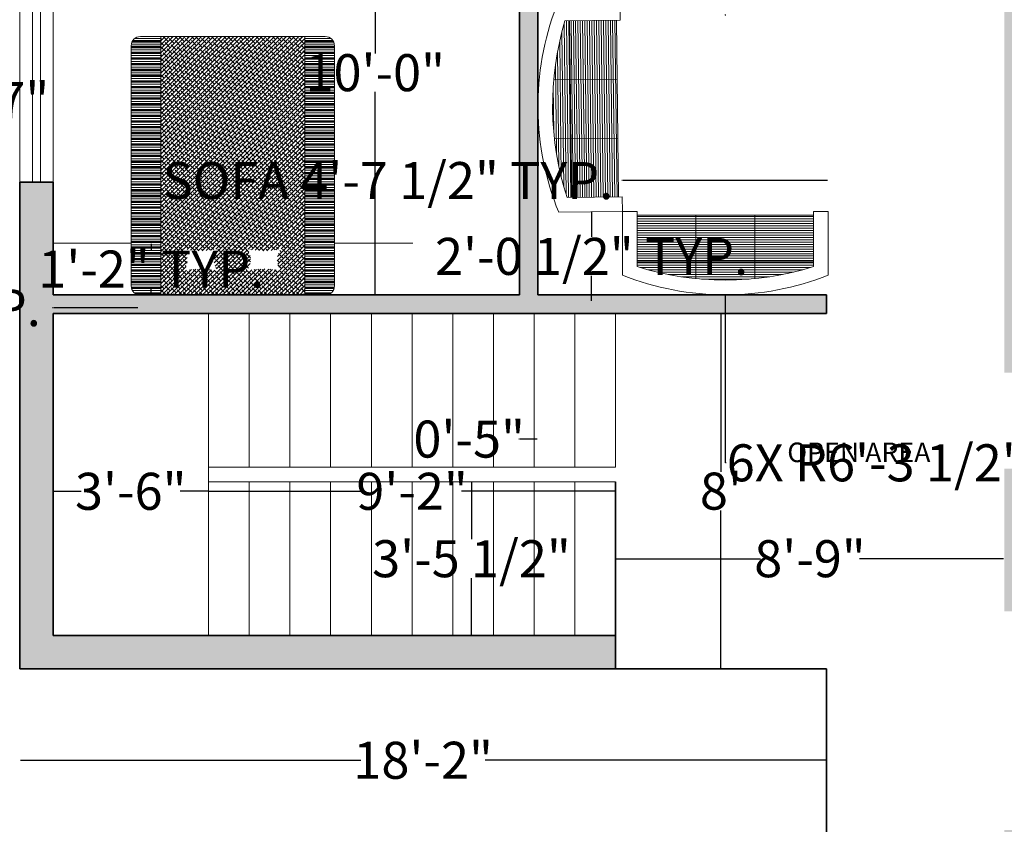
# Model space of a CAD drawing. Units: inches. Extents: x 1198 to 8596, y 144 to 930.
# Tile 3 of 5: x 1348 to 1614, y 536 to 753. Entities that reach past the tile are written whole.
import ezdxf

# ---------------------------------------------------------------- set-up
doc = ezdxf.new("R2010")
doc.units = ezdxf.units.IN
doc.header["$MEASUREMENT"] = 0
doc.layers.get('0').update_dxf_attribs({"color": 50})
for name, color, linetype, lineweight in [('A-ANNO-DIMS', 7, 'Continuous', 18), ('A-AREA-IDEN', 7, 'Continuous', 18), ('A-FLOR-STRS', 120, 'Continuous', 18), ('A-FURN', 11, 'Continuous', 18), ('A-FURN-PATT', 11, 'Continuous', 13), ('A-WALL-PATT', 150, 'Continuous', 13), ('WALL', 7, 'Continuous', 35), ('WINDOW', 2, 'Continuous', 18)]:
    doc.layers.add(name, color=color, linetype=linetype, lineweight=lineweight)
doc.styles.get("Standard").update_dxf_attribs({"font": 'arial.ttf'})
doc.dimstyles.get("Standard").update_dxf_attribs({"dimtxt": 10, "dimasz": 0.18, "dimexe": 0.18, "dimexo": 0.0625, "dimgap": 0.09, "dimtad": 0, "dimtih": 1, "dimtoh": 1, "dimdec": 0, "dimzin": 0, "dimdsep": 46, "dimlunit": 3, "dimtxsty": 'Standard', "dimcen": 0.09, "dimse1": 1, "dimse2": 1, "dimadec": 0, "dimazin": 0, "dimtfac": 1, "dimtdec": 0, "dimtofl": 0, "dimtmove": 0, "dimatfit": 3, "dimfxl": 1, "dimtolj": 1, "dimtzin": 0, "dimarcsym": 0})

# ---------------------------------------------------------------- blocks, each defined once
blk = doc.blocks.new('*D2')
at = {"layer": 'A-ANNO-DIMS', "color": 0, "lineweight": -2, "transparency": 16777216}
for p, q in [((1509.07, 607.65), (1548, 607.65)), ((1613.71, 607.65), (1574.77, 607.65))]:
    blk.add_line(p, q, dxfattribs=at)
at = {"layer": 'A-ANNO-DIMS', "color": 0, "transparency": 16777216}
for points in [[(1509.07, 607.68), (1509.07, 607.62), (1508.89, 607.65)], [(1613.71, 607.68), (1613.71, 607.62), (1613.89, 607.65)]]:
    blk.add_solid(points, dxfattribs=at)
at = {"layer": 'Defpoints', "color": 0, "transparency": 16777216}
for p in [(1508.89, 607.65), (1613.89, 607.65), (1613.89, 607.65)]:
    blk.add_point(p, dxfattribs=at)
at = {"layer": 'A-ANNO-DIMS', "color": 0, "transparency": 16777216, "insert": (1561.39, 607.65), "char_height": 10, "attachment_point": 5}
blk.add_mtext('\\A1;8\'-9"', dxfattribs=at)
blk = doc.blocks.new('*D3')
at = {"layer": 'A-ANNO-DIMS', "color": 0, "lineweight": -2, "transparency": 16777216}
for p, q in [((1537.33, 673.72), (1537.33, 631.09)), ((1537.33, 578.08), (1537.33, 620.7))]:
    blk.add_line(p, q, dxfattribs=at)
at = {"layer": 'A-ANNO-DIMS', "color": 0, "transparency": 16777216}
for points in [[(1537.3, 673.72), (1537.36, 673.72), (1537.33, 673.9)], [(1537.3, 578.08), (1537.36, 578.08), (1537.33, 577.9)]]:
    blk.add_solid(points, dxfattribs=at)
at = {"layer": 'Defpoints', "color": 0, "transparency": 16777216}
for p in [(1537.33, 673.9), (1537.33, 577.9), (1537.33, 577.9)]:
    blk.add_point(p, dxfattribs=at)
at = {"layer": 'A-ANNO-DIMS', "color": 0, "transparency": 16777216, "insert": (1537.33, 625.9), "char_height": 10, "attachment_point": 5}
blk.add_mtext("\\A1;8'", dxfattribs=at)
blk = doc.blocks.new('WD_WIN4')
for p, q in [((-0.5, 0.5), (0.5, 0.5)), ((-0.5, 0.12), (0.5, 0.12)), ((-0.5, -0.12), (0.5, -0.12)), ((-0.5, -0.5), (0.5, -0.5))]:
    blk.add_line(p, q)
blk = doc.blocks.new('Sofa - Roundback 7 ft.')
for p, q in [((-12.00002, -32.4421), (-12.00003, -6.5971)), ((11.99997, -32.4421), (11.99998, -6.5971)), ((-36.000027, -34), (-36.000027, -11.4696)), ((35.99998, -34), (35.99998, -11.4696)), ((-35.999844, -13.3819), (35.9998, -13.3819)), ((-36.000027, -32.4421), (35.99998, -32.4421))]:
    blk.add_line(p, q)
for points in [[(-36.000027, -34), (-42.000027, -34), (-42.000027, -8)], [(41.99998, -8), (41.99998, -34), (35.99998, -34)]]:
    blk.add_lwpolyline(points)
for centre, radius, start, end in [((0, -114.25), 114.25, 68.43141, 111.5686), ((-0.00001, -127.1968), 121.1968, 72.72033, 107.2797)]:
    blk.add_arc(centre, radius, start, end)
blk = doc.blocks.new('*D16')
at = {"layer": 'A-ANNO-DIMS', "color": 0, "lineweight": -2, "transparency": 16777216}
for p, q in [((1337.03, 884.72), (1337.03, 736.59)), ((1337.03, 578.08), (1337.03, 726.2))]:
    blk.add_line(p, q, dxfattribs=at)
at = {"layer": 'A-ANNO-DIMS', "color": 0, "transparency": 16777216}
for points in [[(1337, 884.72), (1337.06, 884.72), (1337.03, 884.9)], [(1337, 578.08), (1337.06, 578.08), (1337.03, 577.9)]]:
    blk.add_solid(points, dxfattribs=at)
at = {"layer": 'Defpoints', "color": 0, "transparency": 16777216}
for p in [(1347.89, 884.9), (1337.03, 577.9), (1347.89, 577.9)]:
    blk.add_point(p, dxfattribs=at)
at = {"layer": 'A-ANNO-DIMS', "color": 0, "transparency": 16777216, "insert": (1337.03, 731.4), "char_height": 10, "attachment_point": 5}
blk.add_mtext('\\A1;25\'-7"', dxfattribs=at)
blk = doc.blocks.new('*D17')
at = {"layer": 'A-ANNO-DIMS', "color": 0, "lineweight": -2, "transparency": 16777216}
for p, q in [((1288.75, 884.72), (1288.75, 551.09)), ((1288.75, 207.08), (1288.75, 540.7))]:
    blk.add_line(p, q, dxfattribs=at)
at = {"layer": 'A-ANNO-DIMS', "color": 0, "transparency": 16777216}
for points in [[(1288.72, 884.72), (1288.78, 884.72), (1288.75, 884.9)], [(1288.72, 207.08), (1288.78, 207.08), (1288.75, 206.9)]]:
    blk.add_solid(points, dxfattribs=at)
at = {"layer": 'Defpoints', "color": 0, "transparency": 16777216}
for p in [(1347.89, 884.9), (1288.75, 206.9), (1347.89, 206.9)]:
    blk.add_point(p, dxfattribs=at)
at = {"layer": 'A-ANNO-DIMS', "color": 0, "transparency": 16777216, "insert": (1288.75, 545.9), "char_height": 10, "attachment_point": 5}
blk.add_mtext('\\A1;56\'-6"', dxfattribs=at)
blk = doc.blocks.new('*D18')
at = {"layer": 'A-ANNO-DIMS', "color": 0, "lineweight": -2, "transparency": 16777216}
for p, q in [((1348.07, 553.22), (1440.09, 553.22)), ((1565.71, 553.22), (1473.68, 553.22))]:
    blk.add_line(p, q, dxfattribs=at)
at = {"layer": 'A-ANNO-DIMS', "color": 0, "transparency": 16777216}
for points in [[(1348.07, 553.25), (1348.07, 553.19), (1347.89, 553.22)], [(1565.71, 553.25), (1565.71, 553.19), (1565.89, 553.22)]]:
    blk.add_solid(points, dxfattribs=at)
at = {"layer": 'Defpoints', "color": 0, "transparency": 16777216}
for p in [(1347.89, 577.9), (1565.89, 577.9), (1565.89, 553.22)]:
    blk.add_point(p, dxfattribs=at)
at = {"layer": 'A-ANNO-DIMS', "color": 0, "transparency": 16777216, "insert": (1456.89, 553.22), "char_height": 10, "attachment_point": 5}
blk.add_mtext('\\A1;18\'-2"', dxfattribs=at)
blk = doc.blocks.new('NIGHTSTAND')
for p, q in [((23.07, 13.96), (0, 13.96)), ((23.07, 0), (23.07, 13.96)), ((1.94, 0), (23.07, 0))]:
    blk.add_line(p, q)
blk = doc.blocks.new('*D26')
at = {"layer": 'A-ANNO-DIMS', "color": 0, "lineweight": -2, "transparency": 16777216}
for p, q in [((1510.72, 709.76), (1510.54, 709.76)), ((1566.15, 709.76), (1510.9, 709.76))]:
    blk.add_line(p, q, dxfattribs=at)
at = {"layer": 'A-ANNO-DIMS', "color": 0, "transparency": 16777216}
for points in [[(1510.9, 709.79), (1510.9, 709.73), (1510.72, 709.76)], [(1566.15, 709.79), (1566.15, 709.73), (1566.33, 709.76)]]:
    blk.add_solid(points, dxfattribs=at)
at = {"layer": 'Defpoints', "color": 0, "transparency": 16777216}
for p in [(1510.72, 709.76), (1510.72, 701.42), (1566.33, 701.42)]:
    blk.add_point(p, dxfattribs=at)
at = {"layer": 'A-ANNO-DIMS', "color": 0, "transparency": 16777216, "insert": (1447.39, 709.76), "char_height": 10, "attachment_point": 5}
blk.add_mtext('\\A1;SOFA 4\'-7 1/2" TYP.', dxfattribs=at)
blk = doc.blocks.new('*D27')
at = {"layer": 'A-ANNO-DIMS', "color": 0, "lineweight": -2, "transparency": 16777216}
for p, q in [((1502.38, 701.24), (1502.38, 694.55)), ((1502.38, 677.33), (1502.38, 684.03))]:
    blk.add_line(p, q, dxfattribs=at)
at = {"layer": 'A-ANNO-DIMS', "color": 0, "transparency": 16777216}
for points in [[(1502.35, 701.24), (1502.41, 701.24), (1502.38, 701.42)], [(1502.35, 677.33), (1502.41, 677.33), (1502.38, 677.15)]]:
    blk.add_solid(points, dxfattribs=at)
at = {"layer": 'Defpoints', "color": 0, "transparency": 16777216}
for p in [(1510.72, 701.42), (1502.38, 677.15), (1510.72, 677.15)]:
    blk.add_point(p, dxfattribs=at)
at = {"layer": 'A-ANNO-DIMS', "color": 0, "transparency": 16777216, "insert": (1502.38, 689.29), "char_height": 10, "attachment_point": 5}
blk.add_mtext('\\A1;2\'-0 1/2" TYP.', dxfattribs=at)
blk = doc.blocks.new('*D28')
at = {"layer": 'A-ANNO-DIMS', "color": 0, "lineweight": -2, "transparency": 16777216}
for p, q in [((1356.89, 675.44), (1356.71, 675.44)), ((1379.78, 675.44), (1357.07, 675.44))]:
    blk.add_line(p, q, dxfattribs=at)
at = {"layer": 'A-ANNO-DIMS', "color": 0, "transparency": 16777216}
for points in [[(1357.07, 675.47), (1357.07, 675.41), (1356.89, 675.44)], [(1379.78, 675.47), (1379.78, 675.41), (1379.96, 675.44)]]:
    blk.add_solid(points, dxfattribs=at)
at = {"layer": 'Defpoints', "color": 0, "transparency": 16777216}
for p in [(1356.89, 678.9), (1379.96, 678.9), (1356.89, 675.44)]:
    blk.add_point(p, dxfattribs=at)
at = {"layer": 'A-ANNO-DIMS', "color": 0, "transparency": 16777216, "insert": (1275.15, 675.44), "char_height": 10, "attachment_point": 5}
blk.add_mtext('\\A1;NIGHTSTAND 1\'-11" TYP.', dxfattribs=at)
blk = doc.blocks.new('*D29')
at = {"layer": 'A-ANNO-DIMS', "color": 0, "lineweight": -2, "transparency": 16777216}
for p, q in [((1383.42, 692.67), (1383.42, 690.99)), ((1383.42, 679.08), (1383.42, 680.76))]:
    blk.add_line(p, q, dxfattribs=at)
at = {"layer": 'A-ANNO-DIMS', "color": 0, "transparency": 16777216}
for points in [[(1383.39, 692.67), (1383.45, 692.67), (1383.42, 692.85)], [(1383.39, 679.08), (1383.45, 679.08), (1383.42, 678.9)]]:
    blk.add_solid(points, dxfattribs=at)
at = {"layer": 'Defpoints', "color": 0, "transparency": 16777216}
for p in [(1379.96, 692.85), (1379.96, 678.9), (1383.42, 678.9)]:
    blk.add_point(p, dxfattribs=at)
at = {"layer": 'A-ANNO-DIMS', "color": 0, "transparency": 16777216, "insert": (1383.42, 685.87), "char_height": 10, "attachment_point": 5}
blk.add_mtext('\\A1;1\'-2" TYP.', dxfattribs=at)
blk = doc.blocks.new('*D38')
at = {"layer": 'A-ANNO-DIMS', "color": 0, "lineweight": -2, "transparency": 16777216}
for p, q in [((1443.94, 798.72), (1443.94, 744.09)), ((1443.94, 679.08), (1443.94, 733.7))]:
    blk.add_line(p, q, dxfattribs=at)
at = {"layer": 'A-ANNO-DIMS', "color": 0, "transparency": 16777216}
for points in [[(1443.91, 798.72), (1443.97, 798.72), (1443.94, 798.9)], [(1443.91, 679.08), (1443.97, 679.08), (1443.94, 678.9)]]:
    blk.add_solid(points, dxfattribs=at)
at = {"layer": 'Defpoints', "color": 0, "transparency": 16777216}
for p in [(1443.94, 798.9), (1482.89, 798.9), (1482.89, 678.9)]:
    blk.add_point(p, dxfattribs=at)
at = {"layer": 'A-ANNO-DIMS', "color": 0, "transparency": 16777216, "insert": (1443.94, 738.9), "char_height": 10, "attachment_point": 5}
blk.add_mtext('\\A1;10\'-0"', dxfattribs=at)
blk = doc.blocks.new('*D39')
at = {"layer": 'A-ANNO-DIMS', "color": 0, "lineweight": -2, "transparency": 16777216}
for p, q in [((1399.07, 625.85), (1440.5, 625.85)), ((1508.71, 625.85), (1467.27, 625.85))]:
    blk.add_line(p, q, dxfattribs=at)
at = {"layer": 'A-ANNO-DIMS', "color": 0, "transparency": 16777216}
for points in [[(1399.07, 625.88), (1399.07, 625.82), (1398.89, 625.85)], [(1508.71, 625.88), (1508.71, 625.82), (1508.89, 625.85)]]:
    blk.add_solid(points, dxfattribs=at)
at = {"layer": 'Defpoints', "color": 0, "transparency": 16777216}
for p in [(1508.89, 625.85), (1398.89, 586.9), (1508.89, 586.9)]:
    blk.add_point(p, dxfattribs=at)
at = {"layer": 'A-ANNO-DIMS', "color": 0, "transparency": 16777216, "insert": (1453.89, 625.85), "char_height": 10, "attachment_point": 5}
blk.add_mtext('\\A1;9\'-2"', dxfattribs=at)
blk = doc.blocks.new('*D40')
at = {"layer": 'A-ANNO-DIMS', "color": 0, "lineweight": -2, "transparency": 16777216}
for p, q in [((1357.07, 625.85), (1364.51, 625.85)), ((1398.71, 625.85), (1391.26, 625.85))]:
    blk.add_line(p, q, dxfattribs=at)
at = {"layer": 'A-ANNO-DIMS', "color": 0, "transparency": 16777216}
for points in [[(1357.07, 625.88), (1357.07, 625.82), (1356.89, 625.85)], [(1398.71, 625.88), (1398.71, 625.82), (1398.89, 625.85)]]:
    blk.add_solid(points, dxfattribs=at)
at = {"layer": 'Defpoints', "color": 0, "transparency": 16777216}
for p in [(1398.89, 625.85), (1356.89, 586.9), (1398.89, 586.9)]:
    blk.add_point(p, dxfattribs=at)
at = {"layer": 'A-ANNO-DIMS', "color": 0, "transparency": 16777216, "insert": (1377.89, 625.85), "char_height": 10, "attachment_point": 5}
blk.add_mtext('\\A1;3\'-6"', dxfattribs=at)
blk = doc.blocks.new('*D41')
at = {"layer": 'A-ANNO-DIMS', "color": 0, "lineweight": -2, "transparency": 16777216}
for p, q in [((1469.94, 628.22), (1469.94, 612.91)), ((1469.94, 587.08), (1469.94, 602.38))]:
    blk.add_line(p, q, dxfattribs=at)
at = {"layer": 'A-ANNO-DIMS', "color": 0, "transparency": 16777216}
for points in [[(1469.91, 628.22), (1469.97, 628.22), (1469.94, 628.4)], [(1469.91, 587.08), (1469.97, 587.08), (1469.94, 586.9)]]:
    blk.add_solid(points, dxfattribs=at)
at = {"layer": 'Defpoints', "color": 0, "transparency": 16777216}
for p in [(1469.94, 628.4), (1508.89, 628.4), (1508.89, 586.9)]:
    blk.add_point(p, dxfattribs=at)
at = {"layer": 'A-ANNO-DIMS', "color": 0, "transparency": 16777216, "insert": (1469.94, 607.65), "char_height": 10, "attachment_point": 5}
blk.add_mtext('\\A1;3\'-5 1/2"', dxfattribs=at)
blk = doc.blocks.new('*D54')
at = {"layer": 'A-ANNO-DIMS', "color": 0, "lineweight": -2, "transparency": 16777216}
for p, q in [((1308.94, 626.78), (1308.94, 597.25)), ((1308.94, 557.33), (1308.94, 586.85))]:
    blk.add_line(p, q, dxfattribs=at)
at = {"layer": 'A-ANNO-DIMS', "color": 0, "transparency": 16777216}
for points in [[(1308.91, 626.78), (1308.97, 626.78), (1308.94, 626.96)], [(1308.91, 557.33), (1308.97, 557.33), (1308.94, 557.15)]]:
    blk.add_solid(points, dxfattribs=at)
at = {"layer": 'Defpoints', "color": 0, "transparency": 16777216}
for p in [(1308.94, 626.96), (1802.33, 626.96), (1802.33, 557.15)]:
    blk.add_point(p, dxfattribs=at)
at = {"layer": 'A-ANNO-DIMS', "color": 0, "transparency": 16777216, "insert": (1308.94, 592.05), "char_height": 10, "attachment_point": 5}
blk.add_mtext('\\A1;5\'-10"', dxfattribs=at)
blk = doc.blocks.new('*D68')
at = {"layer": 'A-ANNO-DIMS', "color": 0, "lineweight": -2, "transparency": 16777216}
for p, q in [((1482.89, 639.95), (1482.71, 639.95)), ((1487.71, 639.95), (1483.07, 639.95))]:
    blk.add_line(p, q, dxfattribs=at)
at = {"layer": 'A-ANNO-DIMS', "color": 0, "transparency": 16777216}
for points in [[(1483.07, 639.98), (1483.07, 639.92), (1482.89, 639.95)], [(1487.71, 639.98), (1487.71, 639.92), (1487.89, 639.95)]]:
    blk.add_solid(points, dxfattribs=at)
at = {"layer": 'Defpoints', "color": 0, "transparency": 16777216}
for p in [(1482.89, 678.9), (1487.89, 678.9), (1482.89, 639.95)]:
    blk.add_point(p, dxfattribs=at)
at = {"layer": 'A-ANNO-DIMS', "color": 0, "transparency": 16777216, "insert": (1469.32, 639.95), "char_height": 10, "attachment_point": 5}
blk.add_mtext('\\A1;0\'-5"', dxfattribs=at)
blk = doc.blocks.new('*D69')
at = {"layer": 'A-ANNO-DIMS', "color": 0, "lineweight": -2, "transparency": 16777216}
for p, q in [((1538.43, 754.55), (1538.61, 754.55)), ((1538.52, 754.46), (1538.52, 754.64)), ((1538.53, 633.54), (1538.53, 678.74)), ((1538.71, 633.54), (1538.53, 633.54))]:
    blk.add_line(p, q, dxfattribs=at)
at = {"layer": 'A-ANNO-DIMS', "color": 0, "transparency": 16777216}
blk.add_solid([(1538.56, 678.74), (1538.5, 678.74), (1538.53, 678.92)], dxfattribs=at)
at = {"layer": 'Defpoints', "color": 0, "transparency": 16777216}
for p in [(1538.52, 754.55), (1538.53, 678.92)]:
    blk.add_point(p, dxfattribs=at)
at = {"layer": 'A-ANNO-DIMS', "color": 0, "transparency": 16777216, "insert": (1579.29, 633.54), "char_height": 10, "attachment_point": 5}
blk.add_mtext('\\A1;6X R6\'-3 1/2"', dxfattribs=at)

msp = doc.modelspace()

# ---------------------------------------------------------------- hatches: boundary and pattern name
at = {"layer": 'A-FURN-PATT'}
h = msp.add_hatch(dxfattribs=at)
h.set_pattern_fill('LINE', color=256, scale=5, angle=-89.3197)
h.set_pattern_definition([(270.6803, (790.78874, 2257.74066), (0.62495594, 0.00742075), [])])
h.paths.add_polyline_path([(1509.27, 737.14), (1509.08, 753.02), (1496.46, 752.87), (1496.65, 736.99)])
h.paths.add_polyline_path([(1509.46, 721.25), (1509.27, 737.14), (1496.65, 736.99), (1496.84, 721.1)])
h.paths.add_polyline_path([(1509.64, 705.36), (1509.46, 721.25), (1496.84, 721.1), (1497.03, 705.21)])
h.paths.add_polyline_path([(1495.76, 705.2), (1497.03, 705.21), (1496.84, 721.1), (1492.35, 721.05, 0.050647)])
h.paths.add_polyline_path([(1496.84, 721.1), (1496.65, 736.99), (1492.16, 736.93, 0.049628), (1492.35, 721.05)])
h.paths.add_polyline_path([(1496.65, 736.99), (1496.46, 752.87), (1495.2, 752.86, 0.050647), (1492.16, 736.93)])
h = msp.add_hatch(dxfattribs=at)
h.set_pattern_fill('PLASTI', color=256, scale=6.190048)
h.set_pattern_definition([(0, (104.9537, 267.4466), (0, 1.547512), []), (0, (104.9537, 267.64), (0, 1.547512), []), (0, (104.9537, 267.8335), (0, 1.547512), []), (0, (104.9537, 268.4138), (0, 1.547512), [])])
h.paths.add_polyline_path([(1424.95, 678.84), (1430.45, 678.84, 0.414214), (1432.92, 681.31), (1432.92, 746.17, 0.414214), (1430.45, 748.65), (1424.95, 748.65)])
h.paths.add_polyline_path([(1378.02, 681.31, 0.414214), (1380.5, 678.84), (1386, 678.84), (1386, 748.65), (1380.5, 748.65, 0.414214), (1378.02, 746.17)])
h = msp.add_hatch(dxfattribs=at)
h.set_pattern_fill('ANSI38', color=256, scale=6.190048)
h.set_pattern_definition([(45, (104.9537, 267.4466), (-0.5471281, 0.5471281), []), (135, (104.9537, 267.4466), (-1.6413843, 0.5471281), [1.93439, -1.160634])])
h.paths.add_polyline_path([(1386, 678.84), (1424.95, 678.84), (1424.95, 748.65), (1386, 748.65)])
h.paths.add_polyline_path([(1401.43, 691.35, 0.358285), (1401.43, 685.35, 0.116256), (1392.11, 685.35, 0.358285), (1392.11, 691.35, 0.116256)], flags=16)
h.paths.add_polyline_path([(1409.19, 691.35, 0.116256), (1418.51, 691.35, 0.358285), (1418.51, 685.35, 0.116256), (1409.19, 685.35, 0.358285)], flags=16)
h = msp.add_hatch(dxfattribs=at)
h.set_pattern_fill('LINE', color=256, scale=5)
h.set_pattern_definition([(0, (1.553, 0.01844), (0, 0.625), [])])
h.paths.add_polyline_path([(1530.58, 700.39), (1514.69, 700.39), (1514.69, 687.77), (1530.58, 687.77)])
h.paths.add_polyline_path([(1546.47, 700.39), (1530.58, 700.39), (1530.58, 687.77), (1546.47, 687.77)])
h.paths.add_polyline_path([(1562.36, 700.39), (1546.47, 700.39), (1546.47, 687.77), (1562.36, 687.77)])
h.paths.add_polyline_path([(1562.36, 686.51), (1562.36, 687.77), (1546.47, 687.77), (1546.47, 683.28, 0.050647)])
h.paths.add_polyline_path([(1546.47, 687.77), (1530.58, 687.77), (1530.58, 683.28, 0.049628), (1546.47, 683.28)])
h.paths.add_polyline_path([(1530.58, 687.77), (1514.69, 687.77), (1514.69, 686.51, 0.050647), (1530.58, 683.28)])
at = {"layer": 'A-WALL-PATT'}
h = msp.add_hatch(color=256, dxfattribs=at)
h.dxf.hatch_style = 1
h.paths.add_polyline_path([(1884.89, 495.9), (1884.89, 534.37), (1875.89, 534.37), (1875.89, 500.9), (1823.11, 500.9), (1823.11, 495.9)])
h.paths.add_polyline_path([(1875.89, 593.42), (1884.89, 593.42), (1884.89, 685.87), (1875.89, 685.87), (1875.89, 631.9), (1749.89, 631.9), (1749.89, 766.08), (1744.89, 766.08), (1744.89, 631.97), (1618.79, 631.97), (1613.89, 631.97), (1613.89, 593.42), (1622.89, 593.42), (1622.89, 626.9), (1744.89, 626.9), (1744.89, 537.33), (1749.89, 537.33), (1749.89, 626.9), (1875.89, 626.9)])
h.paths.add_polyline_path([(1884.89, 206.9), (1884.89, 249.37), (1875.89, 249.37), (1875.89, 215.9), (1842.41, 215.9), (1842.41, 206.9)])
h.paths.add_polyline_path([(1783.36, 206.9), (1783.36, 215.9), (1749.89, 215.9), (1749.89, 308.42), (1744.89, 308.42), (1744.89, 215.9), (1713.41, 215.9), (1713.41, 206.9)])
h.paths.add_polyline_path([(1654.36, 206.9), (1654.36, 215.9), (1622.89, 215.9), (1622.89, 249.37), (1613.89, 249.37), (1613.89, 206.9)])
h.paths.add_polyline_path([(1613.89, 334.34), (1622.89, 334.34), (1622.89, 341.9), (1622.89, 368.41), (1613.89, 368.41)])
h.paths.add_polyline_path([(1613.89, 396.47), (1622.89, 396.47), (1622.89, 418.9), (1710.09, 418.9), (1710.09, 400.51), (1709.89, 346.77), (1709.89, 341.9), (1714.89, 341.9), (1714.89, 346.9), (1714.88, 366), (1714.89, 418.9), (1798.89, 418.9), (1798.89, 346.9), (1734.06, 346.9), (1734.07, 343.96), (1734.06, 341.9), (1744.89, 341.9), (1744.89, 334.34), (1749.89, 334.34), (1749.89, 341.9), (1803.93, 341.9), (1803.93, 346.9), (1803.89, 346.9), (1803.89, 418.9), (1884.89, 418.9), (1884.89, 423.9), (1803.89, 423.9), (1803.89, 495.9), (1803.93, 500.9), (1749.89, 500.9), (1749.89, 511.41), (1747.24, 511.41), (1744.89, 511.41), (1744.89, 500.9), (1734.06, 500.9), (1734.06, 495.9), (1798.89, 495.9), (1798.89, 423.9), (1714.89, 423.9), (1714.89, 495.9), (1714.89, 500.9), (1709.89, 500.9), (1709.89, 496.89), (1709.89, 495.9), (1709.89, 423.9), (1622.89, 423.9), (1622.89, 446.07), (1613.89, 446.07)])
h.paths.add_polyline_path([(1613.89, 474.13), (1622.89, 474.13), (1622.89, 495.9), (1645.93, 495.9), (1683.97, 495.9), (1683.89, 500.9), (1648.32, 500.9), (1648.32, 500.88), (1622.41, 500.86), (1618.52, 500.86), (1613.89, 500.9)])
h.paths.add_polyline_path([(1613.89, 526.77), (1613.89, 534.37), (1622.89, 534.37), (1622.89, 526.77, -0.395914), (1648.3, 502.01), (1648.32, 502.01), (1648.32, 500.88), (1622.41, 500.86), (1622.41, 502), (1648.3, 502.01, 0.395914), (1622.89, 526.77)])
h.paths.add_polyline_path([(1875.89, 744.92), (1884.89, 744.92), (1884.89, 803.9), (1823.06, 803.9), (1823.06, 798.9), (1875.89, 798.9)])
h.paths.add_polyline_path([(1798.89, 803.9), (1734.06, 803.9), (1734.06, 802.45), (1734.06, 798.9), (1744.89, 798.9), (1744.89, 792), (1749.89, 792), (1749.89, 798.9), (1803.89, 798.9), (1803.89, 803.9), (1803.89, 884.9), (1774.16, 884.9), (1774.16, 875.9), (1798.89, 875.9)])
h.paths.add_polyline_path([(1746.09, 875.9), (1746.09, 884.9), (1693.91, 884.9), (1693.91, 875.9), (1709.89, 875.9), (1709.89, 803.9), (1709.89, 798.9), (1714.89, 798.9), (1714.89, 803.9), (1714.89, 875.9)])
h.paths.add_polyline_path([(1618.89, 798.9), (1683.96, 798.9), (1683.96, 803.9), (1618.89, 803.9), (1618.89, 875.9), (1634.86, 875.9), (1634.86, 884.9), (1597.91, 884.9), (1597.91, 875.9), (1613.89, 875.9), (1613.89, 803.9), (1548.75, 803.9), (1548.75, 798.9), (1613.89, 798.9), (1613.89, 657.88), (1618.8, 657.88)])
h.paths.add_polyline_path([(1522.89, 875.9), (1538.86, 875.9), (1538.86, 884.9), (1483.76, 884.9), (1483.76, 875.9), (1517.89, 875.9), (1517.89, 803.9), (1517.89, 802.46), (1517.89, 798.9), (1522.89, 798.9), (1522.89, 803.9)], flags=17)
h.paths.add_polyline_path([(1428.89, 884.9), (1428.89, 803.9), (1428.89, 798.9), (1482.89, 798.9), (1482.89, 678.9), (1356.89, 678.9), (1356.89, 709.37), (1347.89, 709.37), (1347.89, 577.9), (1508.89, 577.9), (1508.89, 586.9), (1356.89, 586.9), (1356.89, 673.9), (1565.89, 673.9), (1565.89, 678.9), (1487.89, 678.9), (1487.89, 798.9), (1498.72, 798.9), (1498.72, 803.9), (1433.89, 803.9), (1433.89, 875.9), (1455.69, 875.9), (1455.69, 884.9)])
h.paths.add_polyline_path([(1356.89, 798.9), (1409.72, 798.9), (1409.72, 803.9), (1347.89, 803.9), (1347.89, 768.42), (1356.89, 768.42)], flags=17)
h.paths.add_polyline_path([(1884.89, 346.9), (1823.09, 346.9, -0.008805), (1823.1, 346.22), (1823.11, 343.35), (1823.09, 341.9), (1875.89, 341.9), (1875.89, 308.42), (1884.89, 308.42)])

# ---------------------------------------------------------------- linework, layer by layer
at = {"layer": 'A-FLOR-STRS'}
for p, q in [((1398.89, 586.9), (1398.89, 673.9)), ((1409.89, 632.4), (1409.89, 673.9)), ((1420.89, 632.4), (1420.89, 673.9)), ((1431.89, 673.9), (1431.89, 632.4)), ((1442.89, 632.4), (1442.89, 673.9)), ((1453.89, 632.4), (1453.89, 673.9)), ((1464.89, 632.4), (1464.89, 673.9)), ((1475.89, 632.4), (1475.89, 673.9)), ((1486.89, 632.4), (1486.89, 673.9)), ((1497.89, 632.4), (1497.89, 673.9)), ((1508.89, 632.4), (1508.89, 673.9)), ((1398.89, 632.4), (1508.89, 632.4)), ((1508.89, 628.4), (1398.89, 628.4)), ((1409.89, 586.9), (1409.89, 628.4)), ((1420.89, 586.9), (1420.89, 628.4)), ((1431.89, 628.4), (1431.89, 586.9)), ((1442.89, 586.9), (1442.89, 628.4)), ((1453.89, 586.9), (1453.89, 628.4)), ((1464.89, 586.9), (1464.89, 628.4)), ((1475.89, 586.9), (1475.89, 628.4)), ((1486.89, 586.9), (1486.89, 628.4)), ((1497.89, 586.9), (1497.89, 628.4)), ((1508.89, 586.9), (1508.89, 628.4))]:
    msp.add_line(p, q, dxfattribs=at)
at = {"layer": 'A-FURN'}
for p, q in [((1386, 678.84), (1386, 748.65)), ((1424.95, 678.84), (1424.95, 748.65)), ((1432.92, 692.85), (1454.06, 692.85)), ((1487.89, 688.91), (1487.89, 688.91))]:
    msp.add_line(p, q, dxfattribs=at)
msp.add_lwpolyline([(1380.5, 678.84), (1430.45, 678.84, 0.414214), (1432.92, 681.31), (1432.92, 746.17, 0.414214), (1430.45, 748.65), (1380.5, 748.65, 0.414214), (1378.02, 746.17), (1378.02, 681.31, 0.414214)], format="xyb", close=True, dxfattribs=at)
at = {"layer": 'WALL'}
for p, q in [((1482.89, 678.9), (1482.89, 798.9)), ((1487.89, 678.9), (1487.89, 798.9)), ((1347.89, 577.9), (1347.89, 709.37)), ((1356.89, 709.37), (1347.89, 709.37)), ((1356.89, 678.9), (1356.89, 709.37)), ((1356.89, 678.9), (1482.89, 678.9)), ((1487.89, 678.9), (1565.89, 678.9)), ((1565.89, 678.9), (1565.89, 673.9)), ((1356.89, 673.9), (1565.89, 673.9)), ((1356.89, 586.9), (1356.89, 673.9)), ((1487.89, 673.9), (1565.89, 673.9)), ((1508.89, 628.4), (1508.89, 577.9)), ((1356.89, 586.9), (1508.89, 586.9)), ((1347.89, 577.9), (1565.89, 577.9)), ((1565.89, 577.9), (1565.89, 206.9))]:
    msp.add_line(p, q, dxfattribs=at)

# ---------------------------------------------------------------- block references
at = {"layer": 'A-FURN', "xscale": 0.6619781710857556, "yscale": 0.6619781710857556, "zscale": 0.6619781710857556}
for p, rotation in [((1487.89, 728.94), 90.68030024111884), ((1538.52, 678.92), 179.9999999999996)]:
    msp.add_blockref('Sofa - Roundback 7 ft.', p, dxfattribs=dict(at, rotation=rotation))
at = {"layer": 'A-FURN', "rotation": 180}
msp.add_blockref('NIGHTSTAND', (1379.96, 692.85), dxfattribs=at)
at = {"layer": 'WINDOW', "xscale": 59.05511811023622, "yscale": 9.000000000000227, "zscale": 59.05511811023622, "rotation": 89.99999999999957}
msp.add_blockref('WD_WIN4', (1352.39, 738.9), dxfattribs=at)

# ---------------------------------------------------------------- texts
at = {"layer": 'A-AREA-IDEN'}
msp.add_text(' OPEN AREA', height=5.299, dxfattribs=at).set_placement((1553.63, 633.72))

# ---------------------------------------------------------------- dimensions: what is measured, and where the dimension line sits
at = {"layer": 'A-ANNO-DIMS'}
for base, p1, p2, angle, override, picture, middle in [((1288.75, 206.9), (1347.89, 884.9), (1347.89, 206.9), 90, {"dimclrd": 0, "dimclre": 0, "dimclrt": 0}, '*D17', (1288.75, 545.9)), ((1337.03, 577.9), (1347.89, 884.9), (1347.89, 577.9), 90, {"dimclrd": 0, "dimclre": 0, "dimclrt": 0}, '*D16', (1337.03, 731.4)), ((1443.94, 798.9), (1482.89, 678.9), (1482.89, 798.9), 90, {"dimdec": 1, "dimlfac": 1, "dimrnd": 0, "dimzin": 1, "dimdsep": 46, "dimlunit": 4, "dimfrac": 2}, '*D38', (1443.94, 738.9)), ((1482.89, 639.95), (1487.89, 678.9), (1482.89, 678.9), 180, {"dimdec": 1, "dimlfac": 1, "dimrnd": 0, "dimzin": 1, "dimdsep": 46, "dimlunit": 4, "dimfrac": 2}, '*D68', (1469.32, 639.95)), ((1537.33, 577.9), (1537.33, 673.9), (1537.33, 577.9), 90, {"dimclrd": 0, "dimclre": 0, "dimclrt": 0}, '*D3', (1537.33, 625.9)), ((1398.89, 625.85), (1356.89, 586.9), (1398.89, 586.9), 0, {"dimdec": 1, "dimlfac": 1, "dimrnd": 0, "dimzin": 1, "dimdsep": 46, "dimlunit": 4, "dimfrac": 2}, '*D40', (1377.89, 625.85)), ((1508.89, 625.85), (1398.89, 586.9), (1508.89, 586.9), 0, {"dimdec": 1, "dimlfac": 1, "dimrnd": 0, "dimzin": 1, "dimdsep": 46, "dimlunit": 4, "dimfrac": 2}, '*D39', (1453.89, 625.85)), ((1469.94, 628.4), (1508.89, 586.9), (1508.89, 628.4), 90, {"dimdec": 1, "dimlfac": 1, "dimrnd": 0, "dimzin": 1, "dimdsep": 46, "dimlunit": 4, "dimfrac": 2}, '*D41', (1469.94, 607.65)), ((1308.94, 626.96), (1802.33, 557.15), (1802.33, 626.96), 90, {"dimdec": 1, "dimlfac": 1, "dimrnd": 0, "dimzin": 1, "dimdsep": 46, "dimlunit": 4, "dimfrac": 2}, '*D54', (1308.94, 592.05))]:
    dim = msp.add_linear_dim(base=base, p1=p1, p2=p2, angle=angle, dimstyle='Standard', override=override, dxfattribs=at)
    dim.commit()
    dim.dimension.update_dxf_attribs({"geometry": picture, "text_midpoint": middle})
dim = msp.add_radius_dim(center=(1538.52, 754.55), mpoint=(1538.53, 678.92), text='6X <>', dimstyle='Standard', override={"dimdec": 1, "dimlfac": 1, "dimrnd": 0, "dimzin": 1, "dimdsep": 46, "dimlunit": 4, "dimfrac": 2}, dxfattribs=at)
dim.commit()
dim.dimension.update_dxf_attribs({"geometry": '*D69', "text_midpoint": (1579.29, 633.54), "dimtype": 164})
for base, p1, p2, angle, text, picture, middle in [((1510.72, 709.76), (1566.33, 701.42), (1510.72, 701.42), 180, 'SOFA <> TYP.', '*D26', (1447.39, 709.76)), ((1502.38, 677.15), (1510.72, 701.42), (1510.72, 677.15), 270, '<> TYP.', '*D27', (1502.38, 689.29)), ((1383.4224, 678.8966), (1379.9612, 692.8531), (1379.9612, 678.8966), 270, '<> TYP.', '*D29', (1383.4224, 685.8748)), ((1356.89, 675.44), (1379.96, 678.9), (1356.89, 678.9), 180, 'NIGHTSTAND <> TYP.', '*D28', (1275.15, 675.44))]:
    dim = msp.add_linear_dim(base=base, p1=p1, p2=p2, angle=angle, text=text, dimstyle='Standard', override={"dimdec": 1, "dimlfac": 1, "dimrnd": 0, "dimzin": 1, "dimdsep": 46, "dimlunit": 4, "dimfrac": 2}, dxfattribs=at)
    dim.commit()
    dim.dimension.update_dxf_attribs({"geometry": picture, "text_midpoint": middle})
for base, p1, p2, picture, middle in [((1613.89, 607.65), (1508.89, 607.65), (1613.89, 607.65), '*D2', (1561.39, 607.65)), ((1565.89, 553.22), (1347.89, 577.9), (1565.89, 577.9), '*D18', (1456.89, 553.22))]:
    dim = msp.add_linear_dim(base=base, p1=p1, p2=p2, dimstyle='Standard', override={"dimclrd": 0, "dimclre": 0, "dimclrt": 0}, dxfattribs=at)
    dim.commit()
    dim.dimension.update_dxf_attribs({"geometry": picture, "text_midpoint": middle})

doc.saveas('drawing.dxf')
